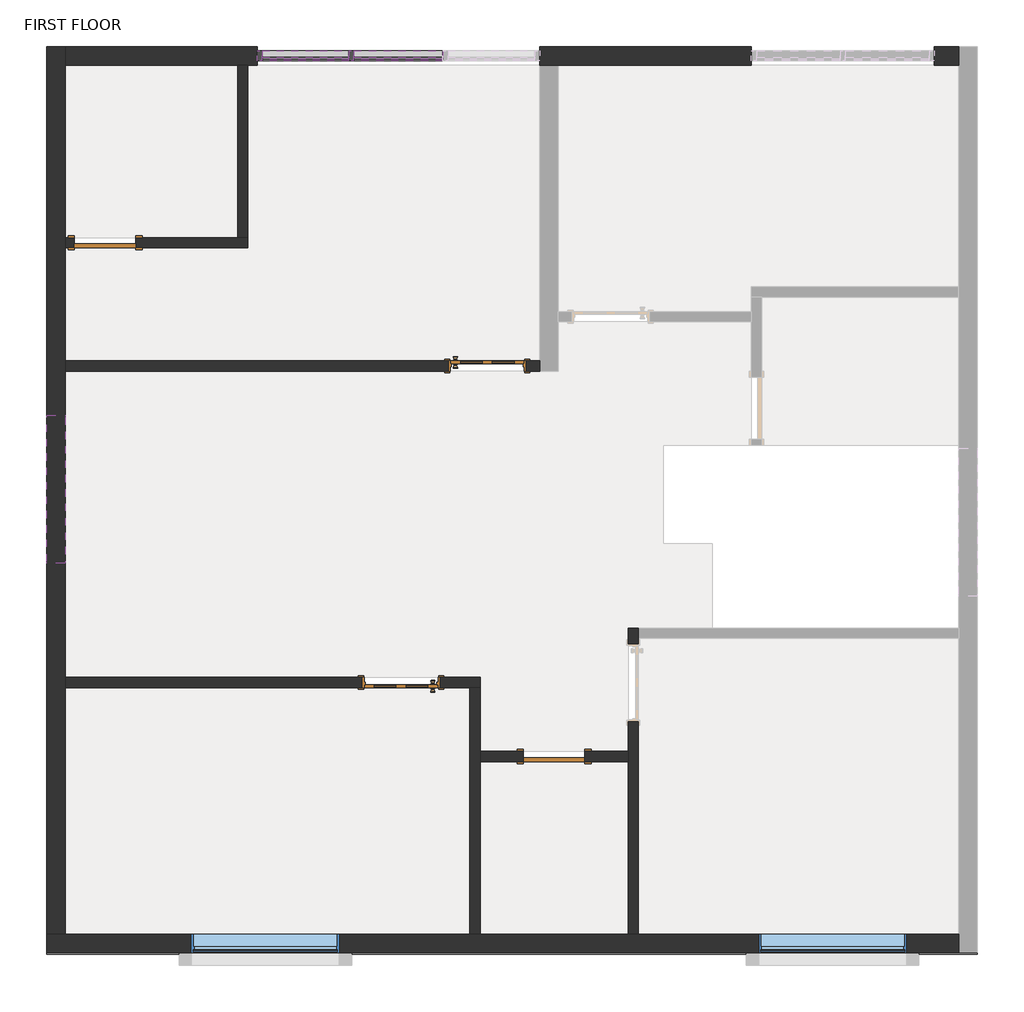
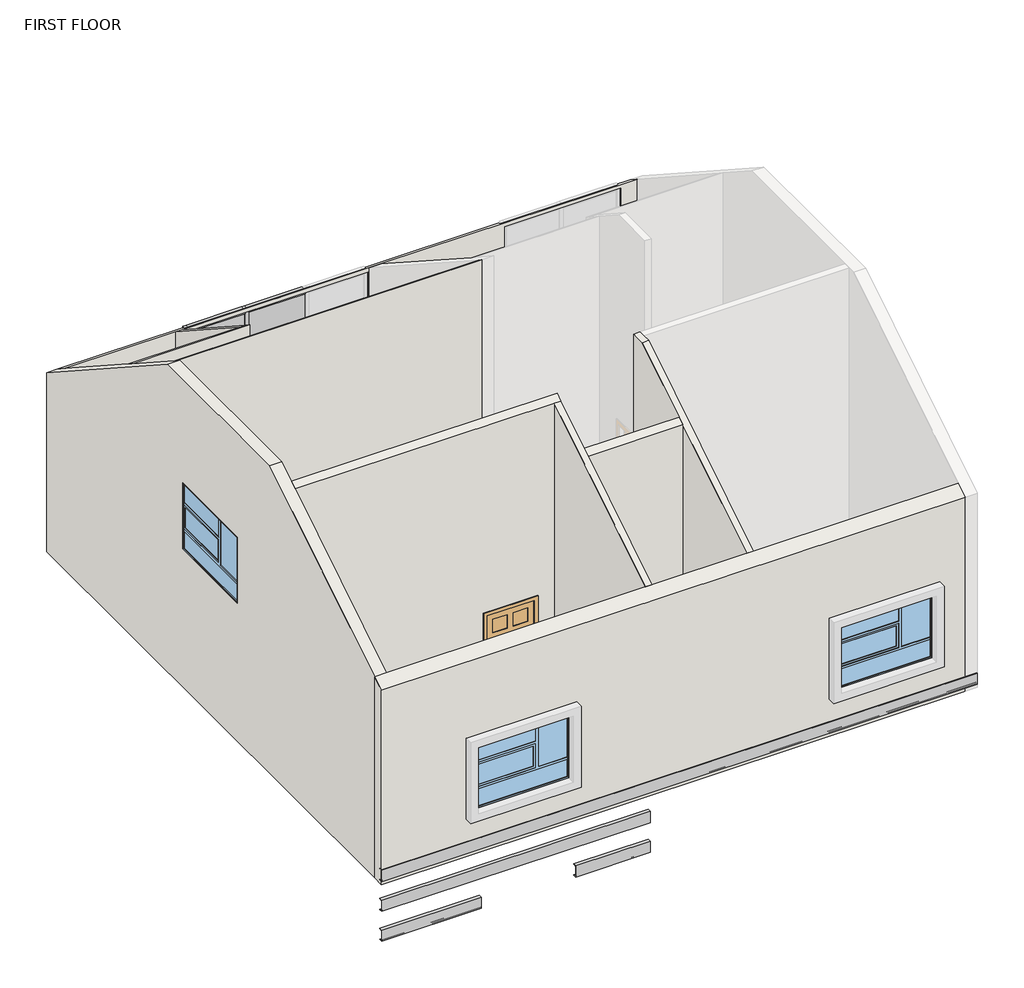
# One storey, part 1 of 2: 17 members, 10 walls, 8 plates, 4 doors, 3 proxies, 3 windows.
"""IFC4 building model written with IfcOpenShell, lengths in millimetres."""

from ifc_helpers import new_model, si_unit, point, frame, frame_2d, origin, place, context, project, spatial, polyline, circle_curve, trimmed, segment, composite_curve, outline, extrude, faceted_brep, transform, mapped, element, save
from ifc_brep_helpers import plane_surface, cylinder_surface, revolved_surface, advanced_brep
from components import door_03e3dfb5, door_1fe7f57d, member_693dcaa1, member_240932ed, member_6e77e263, member_4194b792, member_c45b528a, member_47bfaf8a, member_2b49869a, member_75074519, member_15f4dda0, member_2a4e9e33, system_panel_glazed_03e0ee66, system_panel_glazed_4b7b4477, system_panel_glazed_4d72b045, system_panel_glazed_46ac4994, system_panel_glazed_e581be51, system_panel_glazed_3a317166, system_panel_glazed_99f7726d, system_panel_glazed_de674e10, window_dd9b4f56

model = new_model("IFC4")

# Units and contexts
model_context = context("Model", 3, world=origin())
ifc_project = project(units=[si_unit("LENGTHUNIT", "METRE", prefix="MILLI")], contexts=[model_context])

# Site, building, storey
site = spatial("IfcSite", under=ifc_project)
building = spatial("IfcBuilding", under=site)
storey = spatial("IfcBuildingStorey", under=building, Name="FIRST FLOOR", Elevation=3352.8)

# Proxies
placement = place(None, origin())
element("IfcBuildingElementProxy", 1, Name="Reveal", ObjectType="Reveal", at=placement, inside=storey, context=model_context, shape_type="SweptSolid", body=[
    extrude(outline(composite_curve([segment(polyline([(-2464.7620789, 2433.713469), (-2401.5160789, 2433.713469), (-2401.5160789, 2432.3337932)]), True, "CONTINUOUS"), segment(trimmed(circle_curve(frame_2d((-2406.7611789, 2432.3337932)), 5.2451), [point((-2401.5160789, 2432.3337932))], [point((-2405.8988881, 2427.1600587))], False, "CARTESIAN"), True, "CONTINUOUS"), segment(polyline([(-2405.8988881, 2427.1600587), (-2429.5195789, 2423.223269), (-2448.7574605, 2420.016949)]), True, "CONTINUOUS"), segment(trimmed(circle_curve(frame_2d((-2447.0328789, 2409.66948)), 10.4902), [point((-2448.7574605, 2420.016949))], [point((-2457.5230789, 2409.66948))], True, "CARTESIAN"), True, "CONTINUOUS"), segment(polyline([(-2457.5230789, 2409.66948), (-2457.5230789, 2229.157458)]), True, "CONTINUOUS"), segment(trimmed(circle_curve(frame_2d((-2447.0328789, 2229.157458)), 10.4902), [point((-2457.5230789, 2229.157458))], [point((-2448.7574605, 2218.809989))], True, "CARTESIAN"), True, "CONTINUOUS"), segment(polyline([(-2448.7574605, 2218.809989), (-2429.5195789, 2215.603669), (-2405.8988881, 2211.6668793)]), True, "CONTINUOUS"), segment(trimmed(circle_curve(frame_2d((-2406.7611789, 2206.4931449)), 5.2451), [point((-2405.8988881, 2211.6668793))], [point((-2401.5160789, 2206.4931449))], False, "CARTESIAN"), True, "CONTINUOUS"), segment(polyline([(-2401.5160789, 2206.4931449), (-2401.5160789, 2205.113469), (-2464.7620789, 2205.113469), (-2464.7620789, 2433.713469)]), True, "CONTINUOUS")], self_intersect=False)), frame((-2097.5328791, 0.0, 0.0), z_axis=(1.0, 0.0, 0.0), x_axis=(0.0, 1.0, 0.0)), (0.0, 0.0, 1.0), 1435.1),
    extrude(outline(composite_curve([segment(polyline([(-2464.7620789, 2433.713469), (-2401.5160789, 2433.713469), (-2401.5160789, 2432.3337932)]), True, "CONTINUOUS"), segment(trimmed(circle_curve(frame_2d((-2406.7611789, 2432.3337932)), 5.2451), [point((-2401.5160789, 2432.3337932))], [point((-2405.8988881, 2427.1600587))], False, "CARTESIAN"), True, "CONTINUOUS"), segment(polyline([(-2405.8988881, 2427.1600587), (-2429.5195789, 2423.223269), (-2448.7574605, 2420.016949)]), True, "CONTINUOUS"), segment(trimmed(circle_curve(frame_2d((-2447.0328789, 2409.66948)), 10.4902), [point((-2448.7574605, 2420.016949))], [point((-2457.5230789, 2409.66948))], True, "CARTESIAN"), True, "CONTINUOUS"), segment(polyline([(-2457.5230789, 2409.66948), (-2457.5230789, 2229.157458)]), True, "CONTINUOUS"), segment(trimmed(circle_curve(frame_2d((-2447.0328789, 2229.157458)), 10.4902), [point((-2457.5230789, 2229.157458))], [point((-2448.7574605, 2218.809989))], True, "CARTESIAN"), True, "CONTINUOUS"), segment(polyline([(-2448.7574605, 2218.809989), (-2429.5195789, 2215.603669), (-2405.8988881, 2211.6668793)]), True, "CONTINUOUS"), segment(trimmed(circle_curve(frame_2d((-2406.7611789, 2206.4931449)), 5.2451), [point((-2405.8988881, 2211.6668793))], [point((-2401.5160789, 2206.4931449))], False, "CARTESIAN"), True, "CONTINUOUS"), segment(polyline([(-2401.5160789, 2206.4931449), (-2401.5160789, 2205.113469), (-2464.7620789, 2205.113469), (-2464.7620789, 2433.713469)]), True, "CONTINUOUS")], self_intersect=False)), frame((-5844.0328791, 0.0, 0.0), z_axis=(1.0, 0.0, 0.0), x_axis=(0.0, 1.0, 0.0)), (0.0, 0.0, 1.0), 1917.7),
])
element("IfcBuildingElementProxy", 2, Name="Reveal", ObjectType="Reveal", at=placement, inside=storey, context=model_context, shape_type="SweptSolid", body=[
    extrude(outline(composite_curve([segment(polyline([(-2464.7620789, 3043.313469), (-2401.5160789, 3043.313469), (-2401.5160789, 3041.9337932)]), True, "CONTINUOUS"), segment(trimmed(circle_curve(frame_2d((-2406.7611789, 3041.9337932)), 5.2451), [point((-2401.5160789, 3041.9337932))], [point((-2405.8988881, 3036.7600587))], False, "CARTESIAN"), True, "CONTINUOUS"), segment(polyline([(-2405.8988881, 3036.7600587), (-2429.5195789, 3032.823269), (-2448.7574605, 3029.616949)]), True, "CONTINUOUS"), segment(trimmed(circle_curve(frame_2d((-2447.0328789, 3019.26948)), 10.4902), [point((-2448.7574605, 3029.616949))], [point((-2457.5230789, 3019.26948))], True, "CARTESIAN"), True, "CONTINUOUS"), segment(polyline([(-2457.5230789, 3019.26948), (-2457.5230789, 2838.757458)]), True, "CONTINUOUS"), segment(trimmed(circle_curve(frame_2d((-2447.0328789, 2838.757458)), 10.4902), [point((-2457.5230789, 2838.757458))], [point((-2448.7574605, 2828.409989))], True, "CARTESIAN"), True, "CONTINUOUS"), segment(polyline([(-2448.7574605, 2828.409989), (-2429.5195789, 2825.203669), (-2405.8988881, 2821.2668793)]), True, "CONTINUOUS"), segment(trimmed(circle_curve(frame_2d((-2406.7611789, 2816.0931449)), 5.2451), [point((-2405.8988881, 2821.2668793))], [point((-2401.5160789, 2816.0931449))], False, "CARTESIAN"), True, "CONTINUOUS"), segment(polyline([(-2401.5160789, 2816.0931449), (-2401.5160789, 2814.713469), (-2464.7620789, 2814.713469), (-2464.7620789, 3043.313469)]), True, "CONTINUOUS")], self_intersect=False)), frame((-5844.0328791, 0.0, 0.0), z_axis=(1.0, 0.0, 0.0), x_axis=(0.0, 1.0, 0.0)), (0.0, 0.0, 1.0), 5181.6),
])
element("IfcBuildingElementProxy", 3, Name="Reveal", ObjectType="Reveal", at=placement, inside=storey, context=model_context, shape_type="SweptSolid", body=[
    extrude(outline(composite_curve([segment(polyline([(-2464.7620789, 3652.913469), (-2401.5160789, 3652.913469), (-2401.5160789, 3651.5337932)]), True, "CONTINUOUS"), segment(trimmed(circle_curve(frame_2d((-2406.7611789, 3651.5337932)), 5.2451), [point((-2401.5160789, 3651.5337932))], [point((-2405.8988881, 3646.3600587))], False, "CARTESIAN"), True, "CONTINUOUS"), segment(polyline([(-2405.8988881, 3646.3600587), (-2429.5195789, 3642.423269), (-2448.7574605, 3639.216949)]), True, "CONTINUOUS"), segment(trimmed(circle_curve(frame_2d((-2447.0328789, 3628.86948)), 10.4902), [point((-2448.7574605, 3639.216949))], [point((-2457.5230789, 3628.86948))], True, "CARTESIAN"), True, "CONTINUOUS"), segment(polyline([(-2457.5230789, 3628.86948), (-2457.5230789, 3448.357458)]), True, "CONTINUOUS"), segment(trimmed(circle_curve(frame_2d((-2447.0328789, 3448.357458)), 10.4902), [point((-2457.5230789, 3448.357458))], [point((-2448.7574605, 3438.009989))], True, "CARTESIAN"), True, "CONTINUOUS"), segment(polyline([(-2448.7574605, 3438.009989), (-2429.5195789, 3434.803669), (-2405.8988881, 3430.8668793)]), True, "CONTINUOUS"), segment(trimmed(circle_curve(frame_2d((-2406.7611789, 3425.6931449)), 5.2451), [point((-2405.8988881, 3430.8668793))], [point((-2401.5160789, 3425.6931449))], False, "CARTESIAN"), True, "CONTINUOUS"), segment(polyline([(-2401.5160789, 3425.6931449), (-2401.5160789, 3424.313469), (-2464.7620789, 3424.313469), (-2464.7620789, 3652.913469)]), True, "CONTINUOUS")], self_intersect=False)), frame((-5844.0328791, 0.0, 0.0), z_axis=(1.0, 0.0, 0.0), x_axis=(0.0, 1.0, 0.0)), (0.0, 0.0, 1.0), 11506.2),
])

# Doors
door_shape = door_03e3dfb5(model_context)
element("IfcDoor", 4, ObjectType="Door-Interior-Single-6_Panel-Wood : 36\" x 84\"", at=placement, inside=storey, context=model_context, shape_type="MappedRepresentation", body=[
    mapped(door_shape, transform((-395.7328791, 4804.9973211, 3352.8), x_axis=(1.0, 0.0, 0.0), y_axis=(0.0, 1.0, 0.0), z_axis=(0.0, 0.0, 1.0))),
])
element("IfcDoor", 5, ObjectType="Door-Interior-Single-6_Panel-Wood : 36\" x 84\"", at=placement, inside=storey, context=model_context, shape_type="MappedRepresentation", body=[
    mapped(door_shape, transform((-1462.5328791, 887.0473211, 3352.8), x_axis=(-1.0, 0.0, 0.0), y_axis=(0.0, -1.0, 0.0), z_axis=(0.0, 0.0, 1.0))),
])
door_2_shape = door_1fe7f57d(model_context)
element("IfcDoor", 6, ObjectType="Single-Flush : bathroom flush door 2' 6\" x 7'", at=placement, inside=storey, context=model_context, shape_type="MappedRepresentation", body=[
    mapped(door_2_shape, transform((-5120.1328791, 6325.8223211, 3352.8), x_axis=(-1.0, 0.0, 0.0), y_axis=(0.0, -1.0, 0.0), z_axis=(0.0, 0.0, 1.0))),
])
element("IfcDoor", 7, ObjectType="Single-Flush : bathroom flush door 2' 6\" x 7'", at=placement, inside=storey, context=model_context, shape_type="MappedRepresentation", body=[
    mapped(door_2_shape, transform((429.7671209, -24.1776789, 3352.8), x_axis=(-1.0, 0.0, 0.0), y_axis=(0.0, -1.0, 0.0), z_axis=(0.0, 0.0, 1.0))),
])

# Members
member_shape = member_693dcaa1(model_context)
element("IfcMember", 8, ObjectType="Rectangular Mullion : 2.5\" x 5\" rectangular", at=placement, inside=storey, context=model_context, shape_type="MappedRepresentation", body=[
    mapped(member_shape, transform((-3177.0328791, 8637.2223211, 7085.0688597), x_axis=(0.0, 0.0, 1.0), y_axis=(0.0, 1.0, 0.0), z_axis=(-1.0, 0.0, 0.0))),
])
member_2_shape = member_240932ed(model_context)
element("IfcMember", 9, ObjectType="Rectangular Mullion : 2.5\" x 5\" rectangular", at=placement, inside=storey, context=model_context, shape_type="MappedRepresentation", body=[
    mapped(member_2_shape, transform((-2044.6162124, 8637.2223211, 7085.0688597), x_axis=(0.0, 0.0, 1.0), y_axis=(0.0, 1.0, 0.0), z_axis=(-1.0, 0.0, 0.0))),
])
element("IfcMember", 10, ObjectType="Rectangular Mullion : 2.5\" x 5\" rectangular", at=placement, inside=storey, context=model_context, shape_type="MappedRepresentation", body=[
    mapped(member_shape, transform((-2108.1162124, 8637.2223211, 3352.8), x_axis=(0.0, 0.0, -1.0), y_axis=(0.0, 1.0, 0.0), z_axis=(1.0, 0.0, 0.0))),
])
member_3_shape = member_6e77e263(model_context)
element("IfcMember", 11, ObjectType="Rectangular Mullion : 2.5\" x 5\" rectangular", at=placement, inside=storey, context=model_context, shape_type="MappedRepresentation", body=[
    mapped(member_3_shape, transform((-2076.3662124, 8637.2223211, 3352.8), x_axis=(-1.0, 0.0, 0.0), y_axis=(0.0, 1.0, 0.0), z_axis=(0.0, 0.0, -1.0))),
])
member_4_shape = member_4194b792(model_context)
element("IfcMember", 12, ObjectType="Rectangular Mullion : 2.5\" x 5\" rectangular", at=placement, inside=storey, context=model_context, shape_type="MappedRepresentation", body=[
    mapped(member_4_shape, transform((-3177.0328791, 8637.2223211, 3962.4), x_axis=(0.0, 0.0, 1.0), y_axis=(0.0, 1.0, 0.0), z_axis=(-1.0, 0.0, 0.0))),
])
element("IfcMember", 13, ObjectType="Rectangular Mullion : 2.5\" x 5\" rectangular", at=placement, inside=storey, context=model_context, shape_type="MappedRepresentation", body=[
    mapped(member_4_shape, transform((-3177.0328791, 8637.2223211, 5181.6), x_axis=(0.0, 0.0, 1.0), y_axis=(0.0, 1.0, 0.0), z_axis=(-1.0, 0.0, 0.0))),
])
element("IfcMember", 14, ObjectType="Rectangular Mullion : 2.5\" x 5\" rectangular", at=placement, inside=storey, context=model_context, shape_type="MappedRepresentation", body=[
    mapped(member_4_shape, transform((-3177.0328791, 8637.2223211, 5791.2), x_axis=(0.0, 0.0, 1.0), y_axis=(0.0, 1.0, 0.0), z_axis=(-1.0, 0.0, 0.0))),
])
member_5_shape = member_c45b528a(model_context)
element("IfcMember", 15, ObjectType="Rectangular Mullion : 2.5\" x 5\" rectangular", at=placement, inside=storey, context=model_context, shape_type="MappedRepresentation", body=[
    mapped(member_5_shape, transform((-2044.6162124, 8637.2223211, 3962.4), x_axis=(0.0, 0.0, 1.0), y_axis=(0.0, 1.0, 0.0), z_axis=(-1.0, 0.0, 0.0))),
])
element("IfcMember", 16, ObjectType="Rectangular Mullion : 2.5\" x 5\" rectangular", at=placement, inside=storey, context=model_context, shape_type="MappedRepresentation", body=[
    mapped(member_5_shape, transform((-2044.6162124, 8637.2223211, 5181.6), x_axis=(0.0, 0.0, 1.0), y_axis=(0.0, 1.0, 0.0), z_axis=(-1.0, 0.0, 0.0))),
])
element("IfcMember", 17, ObjectType="Rectangular Mullion : 2.5\" x 5\" rectangular", at=placement, inside=storey, context=model_context, shape_type="MappedRepresentation", body=[
    mapped(member_5_shape, transform((-2044.6162124, 8637.2223211, 5791.2), x_axis=(0.0, 0.0, 1.0), y_axis=(0.0, 1.0, 0.0), z_axis=(-1.0, 0.0, 0.0))),
])
member_6_shape = member_47bfaf8a(model_context)
element("IfcMember", 18, ObjectType="Rectangular Mullion : 2.5\" x 5\" rectangular", at=placement, inside=storey, context=model_context, shape_type="MappedRepresentation", body=[
    mapped(member_6_shape, transform((-3240.5328791, 8637.2223211, 3352.8), x_axis=(-1.0, 0.0, 0.0), y_axis=(0.0, 1.0, 0.0), z_axis=(0.0, 0.0, -1.0))),
])
member_7_shape = member_2b49869a(model_context)
element("IfcMember", 19, ObjectType="Rectangular Mullion : 2.5\" x 5\" rectangular", at=placement, inside=storey, context=model_context, shape_type="MappedRepresentation", body=[
    mapped(member_7_shape, transform((-2076.3662124, 8637.2223211, 3962.4), x_axis=(-1.0, 0.0, 0.0), y_axis=(0.0, 1.0, 0.0), z_axis=(0.0, 0.0, -1.0))),
])
member_8_shape = member_75074519(model_context)
element("IfcMember", 20, ObjectType="Rectangular Mullion : 2.5\" x 5\" rectangular", at=placement, inside=storey, context=model_context, shape_type="MappedRepresentation", body=[
    mapped(member_8_shape, transform((-3240.5328791, 8637.2223211, 3962.4), x_axis=(-1.0, 0.0, 0.0), y_axis=(0.0, 1.0, 0.0), z_axis=(0.0, 0.0, -1.0))),
])
element("IfcMember", 21, ObjectType="Rectangular Mullion : 2.5\" x 5\" rectangular", at=placement, inside=storey, context=model_context, shape_type="MappedRepresentation", body=[
    mapped(member_3_shape, transform((-2076.3662124, 8637.2223211, 5181.6), x_axis=(-1.0, 0.0, 0.0), y_axis=(0.0, 1.0, 0.0), z_axis=(0.0, 0.0, -1.0))),
])
element("IfcMember", 22, ObjectType="Rectangular Mullion : 2.5\" x 5\" rectangular", at=placement, inside=storey, context=model_context, shape_type="MappedRepresentation", body=[
    mapped(member_6_shape, transform((-3240.5328791, 8637.2223211, 5181.6), x_axis=(-1.0, 0.0, 0.0), y_axis=(0.0, 1.0, 0.0), z_axis=(0.0, 0.0, -1.0))),
])
member_9_shape = member_15f4dda0(model_context)
element("IfcMember", 23, ObjectType="Rectangular Mullion : 2.5\" x 5\" rectangular", at=placement, inside=storey, context=model_context, shape_type="MappedRepresentation", body=[
    mapped(member_9_shape, transform((-2076.3662124, 8637.2223211, 5791.2), x_axis=(-1.0, 0.0, 0.0), y_axis=(0.0, 1.0, 0.0), z_axis=(0.0, 0.0, -1.0))),
])
member_10_shape = member_2a4e9e33(model_context)
element("IfcMember", 24, ObjectType="Rectangular Mullion : 2.5\" x 5\" rectangular", at=placement, inside=storey, context=model_context, shape_type="MappedRepresentation", body=[
    mapped(member_10_shape, transform((-3240.5328791, 8637.2223211, 5791.2), x_axis=(-1.0, 0.0, 0.0), y_axis=(0.0, 1.0, 0.0), z_axis=(0.0, 0.0, -1.0))),
])

# Plates
system_panel_glazed_shape = system_panel_glazed_03e0ee66(model_context)
element("IfcPlate", 25, ObjectType="System Panel : Glazed", at=placement, inside=storey, context=model_context, shape_type="MappedRepresentation", body=[
    mapped(system_panel_glazed_shape, transform((-2642.5745458, 8637.2223211, 3416.3), x_axis=(-1.0, 0.0, 0.0), y_axis=(0.0, -1.0, 0.0), z_axis=(0.0, 0.0, 1.0))),
])
system_panel_glazed_2_shape = system_panel_glazed_4b7b4477(model_context)
element("IfcPlate", 26, ObjectType="System Panel : Glazed", at=placement, inside=storey, context=model_context, shape_type="MappedRepresentation", body=[
    mapped(system_panel_glazed_2_shape, transform((-1494.2828791, 8637.2223211, 3416.3), x_axis=(-1.0, 0.0, 0.0), y_axis=(0.0, -1.0, 0.0), z_axis=(0.0, 0.0, 1.0))),
])
system_panel_glazed_3_shape = system_panel_glazed_4d72b045(model_context)
element("IfcPlate", 27, ObjectType="System Panel : Glazed", at=placement, inside=storey, context=model_context, shape_type="MappedRepresentation", body=[
    mapped(system_panel_glazed_3_shape, transform((-1494.2828791, 8637.2223211, 3994.15), x_axis=(-1.0, 0.0, 0.0), y_axis=(0.0, -1.0, 0.0), z_axis=(0.0, 0.0, 1.0))),
])
system_panel_glazed_4_shape = system_panel_glazed_46ac4994(model_context)
element("IfcPlate", 28, ObjectType="System Panel : Glazed", at=placement, inside=storey, context=model_context, shape_type="MappedRepresentation", body=[
    mapped(system_panel_glazed_4_shape, transform((-2642.5745458, 8637.2223211, 3994.15), x_axis=(-1.0, 0.0, 0.0), y_axis=(0.0, -1.0, 0.0), z_axis=(0.0, 0.0, 1.0))),
])
system_panel_glazed_5_shape = system_panel_glazed_e581be51(model_context)
element("IfcPlate", 29, ObjectType="System Panel : Glazed", at=placement, inside=storey, context=model_context, shape_type="MappedRepresentation", body=[
    mapped(system_panel_glazed_5_shape, transform((-2642.5745458, 8637.2223211, 5213.35), x_axis=(-1.0, 0.0, 0.0), y_axis=(0.0, -1.0, 0.0), z_axis=(0.0, 0.0, 1.0))),
])
system_panel_glazed_6_shape = system_panel_glazed_3a317166(model_context)
element("IfcPlate", 30, ObjectType="System Panel : Glazed", at=placement, inside=storey, context=model_context, shape_type="MappedRepresentation", body=[
    mapped(system_panel_glazed_6_shape, transform((-1494.2828791, 8637.2223211, 5213.35), x_axis=(-1.0, 0.0, 0.0), y_axis=(0.0, -1.0, 0.0), z_axis=(0.0, 0.0, 1.0))),
])
system_panel_glazed_7_shape = system_panel_glazed_99f7726d(model_context)
element("IfcPlate", 31, ObjectType="System Panel : Glazed", at=placement, inside=storey, context=model_context, shape_type="MappedRepresentation", body=[
    mapped(system_panel_glazed_7_shape, transform((-2642.5745458, 8637.2223211, 5822.95), x_axis=(-1.0, 0.0, 0.0), y_axis=(0.0, -1.0, 0.0), z_axis=(0.0, 0.0, 1.0))),
])
system_panel_glazed_8_shape = system_panel_glazed_de674e10(model_context)
element("IfcPlate", 32, ObjectType="System Panel : Glazed", at=placement, inside=storey, context=model_context, shape_type="MappedRepresentation", body=[
    mapped(system_panel_glazed_8_shape, transform((-1494.2828791, 8637.2223211, 5822.95), x_axis=(-1.0, 0.0, 0.0), y_axis=(0.0, -1.0, 0.0), z_axis=(0.0, 0.0, 1.0))),
])

# Walls
element("IfcWall", 33, ObjectType="INNER WALL 5\"", at=placement, inside=storey, context=model_context, shape_type="Brep", body=[
    faceted_brep([(-5615.4328791, 6262.3223211, 3352.8), (-5501.1328791, 6262.3223211, 3352.8), (-5501.1328791, 6262.3223211, 5384.8), (-4739.1328791, 6262.3223211, 5384.8), (-4739.1328791, 6262.3223211, 3352.8), (-3354.8328791, 6262.3223211, 3352.8), (-3354.8328791, 6262.3223211, 8627.3469528), (-5615.4328791, 6262.3223211, 8627.3469528), (-5501.1328791, 6389.3223211, 5384.8), (-5501.1328791, 6389.3223211, 3352.8), (-5615.4328791, 6389.3223211, 3352.8), (-5615.4328791, 6389.3223211, 8544.8721884), (-3481.8328791, 6389.3223211, 8544.8721884), (-3354.8328791, 6389.3223211, 8544.8721884), (-3354.8328791, 6389.3223211, 3352.8), (-3481.8328791, 6389.3223211, 3352.8), (-4739.1328791, 6389.3223211, 3352.8), (-4739.1328791, 6389.3223211, 5384.8)], [[[0, 1, 2, 3, 4, 5, 6, 7]], [[8, 9, 10, 11, 12, 13, 14, 15, 16, 17]], [[10, 9, 1, 0]], [[16, 15, 14, 5, 4]], [[0, 7, 11, 10]], [[6, 5, 14, 13]], [[2, 1, 9, 8]], [[3, 2, 8, 17]], [[4, 3, 17, 16]], [[7, 6, 13, 12, 11]]]),
])
element("IfcWall", 34, ObjectType="INNER WALL 5\"", at=placement, inside=storey, context=model_context, shape_type="SweptSolid", body=[
    extrude(outline(polyline([(6389.3223211, 3352.8), (6389.3223211, 8544.8721884), (8522.9223211, 7159.2961476), (8522.9223211, 3352.8), (6389.3223211, 3352.8)])), frame((-3481.8328791, 0.0, 0.0), z_axis=(1.0, 0.0, 0.0), x_axis=(0.0, 1.0, 0.0)), (0.0, 0.0, 1.0), 127.0),
])
element("IfcWall", 35, ObjectType="INNER WALL 5\"", at=placement, inside=storey, context=model_context, shape_type="Brep", body=[
    faceted_brep([(251.9671209, 4738.3223211, 3352.8), (251.9671209, 4738.3223211, 9617.0441248), (-5615.4328791, 4738.3223211, 9617.0441248), (-5615.4328791, 4738.3223211, 3352.8), (-878.3328791, 4738.3223211, 3352.8), (-878.3328791, 4738.3223211, 5511.8), (86.8671209, 4738.3223211, 5511.8), (86.8671209, 4738.3223211, 3352.8), (251.9671209, 4865.3223211, 9534.5693605), (251.9671209, 4865.3223211, 3352.8), (86.8671209, 4865.3223211, 3352.8), (86.8671209, 4865.3223211, 5511.8), (-878.3328791, 4865.3223211, 5511.8), (-878.3328791, 4865.3223211, 3352.8), (-5615.4328791, 4865.3223211, 3352.8), (-5615.4328791, 4865.3223211, 9534.5693605)], [[[0, 1, 2, 3, 4, 5, 6, 7]], [[8, 9, 10, 11, 12, 13, 14, 15]], [[3, 14, 13, 4]], [[9, 0, 7, 10]], [[1, 0, 9, 8]], [[3, 2, 15, 14]], [[6, 11, 10, 7]], [[11, 6, 5, 12]], [[12, 5, 4, 13]], [[2, 1, 8, 15]]]),
])
element("IfcWall", 36, ObjectType="INNER WALL 5\"", at=placement, inside=storey, context=model_context, shape_type="Brep", body=[
    faceted_brep([(1471.1671209, -2221.2776789, 7460.5048127), (1471.1671209, -2221.2776789, 3352.8), (1471.1671209, 407.6223211, 3352.8), (1471.1671209, 407.6223211, 5511.8), (1471.1671209, 1372.8223211, 5511.8), (1471.1671209, 1372.8223211, 3352.8), (1471.1671209, 1436.3223211, 3352.8), (1471.1671209, 1563.3223211, 3352.8), (1471.1671209, 1563.3223211, 9646.3602906), (1471.1671209, 1436.3223211, 9646.3602906), (1471.1671209, 1276.8223179, 9646.3602906), (1344.1671209, -2221.2776789, 3352.8), (1344.1671209, -2221.2776789, 7460.5048127), (1344.1671209, -87.6776789, 8793.726062), (1344.1671209, 39.3223211, 8873.0844697), (1344.1671209, 1276.8223179, 9646.3602906), (1344.1671209, 1563.3223211, 9646.3602906), (1344.1671209, 1563.3223211, 3352.8), (1344.1671209, 1372.8223211, 3352.8), (1344.1671209, 1372.8223211, 5511.8), (1344.1671209, 407.6223211, 5511.8), (1344.1671209, 407.6223211, 3352.8), (1344.1671209, 39.3223211, 3352.8), (1344.1671209, -87.6776789, 3352.8)], [[[0, 1, 2, 3, 4, 5, 6, 7, 8, 9, 10]], [[11, 12, 13, 14, 15, 16, 17, 18, 19, 20, 21, 22, 23]], [[1, 11, 23, 22, 21, 2]], [[17, 7, 6, 5, 18]], [[1, 0, 12, 11]], [[8, 7, 17, 16]], [[20, 3, 2, 21]], [[3, 20, 19, 4]], [[4, 19, 18, 5]], [[12, 0, 10, 15, 14, 13]], [[8, 16, 15, 10, 9]]]),
])
element("IfcWall", 37, ObjectType="INNER WALL 5\"", at=placement, inside=storey, context=model_context, shape_type="Brep", body=[
    faceted_brep([(-5615.4328791, 826.7223211, 9365.1065974), (-5615.4328791, 826.7223211, 3352.8), (-1945.1328791, 826.7223211, 3352.8), (-1945.1328791, 826.7223211, 5511.8), (-979.9328791, 826.7223211, 5511.8), (-979.9328791, 826.7223211, 3352.8), (-611.6328791, 826.7223211, 3352.8), (-484.6328791, 826.7223211, 3352.8), (-484.6328791, 826.7223211, 9365.1065974), (-611.6328791, 826.7223211, 9365.1065974), (-5615.4328791, 953.7223211, 3352.8), (-5615.4328791, 953.7223211, 9444.4650051), (-484.6328791, 953.7223211, 9444.4650051), (-484.6328791, 953.7223211, 3352.8), (-979.9328791, 953.7223211, 3352.8), (-979.9328791, 953.7223211, 5511.8), (-1945.1328791, 953.7223211, 5511.8), (-1945.1328791, 953.7223211, 3352.8)], [[[0, 1, 2, 3, 4, 5, 6, 7, 8, 9]], [[10, 11, 12, 13, 14, 15, 16, 17]], [[1, 10, 17, 2]], [[13, 7, 6, 5, 14]], [[1, 0, 11, 10]], [[8, 7, 13, 12]], [[16, 3, 2, 17]], [[3, 16, 15, 4]], [[4, 15, 14, 5]], [[0, 9, 8, 12, 11]]]),
])
element("IfcWall", 38, ObjectType="INNER WALL 5\"", at=placement, inside=storey, context=model_context, shape_type="Brep", body=[
    faceted_brep([(-611.6328791, 826.7223211, 3352.8), (-611.6328791, -2221.2776789, 3352.8), (-611.6328791, -2221.2776789, 7460.5048127), (-611.6328791, 826.7223211, 9365.1065974), (-484.6328791, 826.7223211, 3352.8), (-484.6328791, 826.7223211, 9365.1065974), (-484.6328791, 39.3223211, 8873.0844697), (-484.6328791, -87.6776789, 8793.726062), (-484.6328791, -2221.2776789, 7460.5048127), (-484.6328791, -2221.2776789, 3352.8), (-484.6328791, -87.6776789, 3352.8), (-484.6328791, 39.3223211, 3352.8)], [[[0, 1, 2, 3]], [[4, 5, 6, 7, 8, 9, 10, 11]], [[1, 0, 4, 11, 10, 9]], [[0, 3, 5, 4]], [[2, 1, 9, 8]], [[3, 2, 8, 7, 6, 5]]]),
])
element("IfcWall", 39, ObjectType="INNER WALL 5\"", at=placement, inside=storey, context=model_context, shape_type="Brep", body=[
    faceted_brep([(-484.6328791, -87.6776789, 3352.8), (48.7671209, -87.6776789, 3352.8), (48.7671209, -87.6776789, 5384.8), (810.7671209, -87.6776789, 5384.8), (810.7671209, -87.6776789, 3352.8), (1344.1671209, -87.6776789, 3352.8), (1344.1671209, -87.6776789, 8793.726062), (-484.6328791, -87.6776789, 8793.726062), (48.7671209, 39.3223211, 5384.8), (48.7671209, 39.3223211, 3352.8), (-484.6328791, 39.3223211, 3352.8), (-484.6328791, 39.3223211, 8873.0844697), (1344.1671209, 39.3223211, 8873.0844697), (1344.1671209, 39.3223211, 3352.8), (810.7671209, 39.3223211, 3352.8), (810.7671209, 39.3223211, 5384.8)], [[[0, 1, 2, 3, 4, 5, 6, 7]], [[8, 9, 10, 11, 12, 13, 14, 15]], [[14, 13, 5, 4]], [[10, 9, 1, 0]], [[6, 5, 13, 12]], [[0, 7, 11, 10]], [[2, 1, 9, 8]], [[3, 2, 8, 15]], [[4, 3, 15, 14]], [[7, 6, 12, 11]]]),
])
element("IfcWall", 40, ObjectType="OUTER WALL 9\"", at=placement, inside=storey, context=model_context, shape_type="AdvancedBrep", body=[
    advanced_brep(
    [(5433.5671209, -2221.2776789, 3352.8), (1471.1671209, -2221.2776789, 3352.8), (1344.1671209, -2221.2776789, 3352.8), (-484.6328791, -2221.2776789, 3352.8), (-611.6328791, -2221.2776789, 3352.8), (-5615.4328791, -2221.2776789, 3352.8), (-5844.0328791, -2221.2776789, 3352.8), (-5844.0328791, -2221.2776789, 7460.5048127), (-5615.4328791, -2221.2776789, 7460.5048127), (-611.6328791, -2221.2776789, 7460.5048127), (-484.6328791, -2221.2776789, 7460.5048127), (1344.1671209, -2221.2776789, 7460.5048127), (1471.1671209, -2221.2776789, 7460.5048127), (5433.5671209, -2221.2776789, 7460.5048127), (-4053.3328791, -2221.2776789, 5613.4), (-4053.3328791, -2221.2776789, 4267.2), (-2224.5328791, -2221.2776789, 4267.2), (-2224.5328791, -2221.2776789, 5613.4), (2957.0671209, -2221.2776789, 5613.4), (2957.0671209, -2221.2776789, 4267.2), (4785.8671209, -2221.2776789, 4267.2), (4785.8671209, -2221.2776789, 5613.4), (-5844.0328791, -2449.8776789, 3352.8), (5433.5671209, -2449.8776789, 3352.8), (5433.5671209, -2449.8776789, 3424.313469), (-5844.0328791, -2449.8776789, 3424.313469), (5433.5671209, -2449.8776789, 7317.6596789), (-5844.0328791, -2449.8776789, 7317.6596789), (-5844.0328791, -2449.8776789, 3652.913469), (5433.5671209, -2449.8776789, 3652.913469), (-4053.3328791, -2449.8776789, 4267.2), (-4053.3328791, -2449.8776789, 5613.4), (-2224.5328791, -2449.8776789, 5613.4), (-2224.5328791, -2449.8776789, 4267.2), (2957.0671209, -2449.8776789, 4267.2), (2957.0671209, -2449.8776789, 5613.4), (4785.8671209, -2449.8776789, 5613.4), (4785.8671209, -2449.8776789, 4267.2), (5433.5671209, -2449.8776789, 3438.260359), (5433.5671209, -2449.8776789, 3638.9665791), (-5844.0328791, -2449.8776789, 3638.9665791), (-5844.0328791, -2449.8776789, 3438.260359), (5433.5671209, -2401.5160789, 3652.913469), (5433.5671209, -2401.5160789, 3651.5337932), (5433.5671209, -2405.8988881, 3646.3600587), (5433.5671209, -2448.7574605, 3639.216949), (5433.5671209, -2448.7574605, 3438.009989), (5433.5671209, -2405.8988881, 3430.8668793), (5433.5671209, -2401.5160789, 3425.6931449), (5433.5671209, -2401.5160789, 3424.313469), (-5844.0328791, -2401.5160789, 3424.313469), (-5844.0328791, -2401.5160789, 3425.6931449), (-5844.0328791, -2405.8988881, 3430.8668793), (-5844.0328791, -2448.7574605, 3438.009989), (-5844.0328791, -2448.7574605, 3639.216949), (-5844.0328791, -2405.8988881, 3646.3600587), (-5844.0328791, -2401.5160789, 3651.5337932), (-5844.0328791, -2401.5160789, 3652.913469)],
    [
        (0, 1),
        (1, 2),
        (2, 3),
        (3, 4),
        (4, 5),
        (5, 6),
        (6, 7),
        (7, 8),
        (8, 9),
        (9, 10),
        (10, 11),
        (11, 12),
        (12, 13),
        (13, 0),
        (14, 15),
        (15, 16),
        (16, 17),
        (17, 14),
        (18, 19),
        (19, 20),
        (20, 21),
        (21, 18),
        (22, 23),
        (23, 24),
        (24, 25),
        (25, 22),
        (26, 27),
        (27, 28),
        (28, 29),
        (29, 26),
        (30, 31),
        (31, 32),
        (32, 33),
        (33, 30),
        (34, 35),
        (35, 36),
        (36, 37),
        (37, 34),
        (38, 39),
        (39, 40),
        (40, 41),
        (41, 38),
        (0, 23),
        (22, 6),
        (13, 26),
        (29, 42),
        (42, 43),
        (43, 44, circle_curve(frame((5433.5671209, -2406.7611789, 3651.5337932), z_axis=(-1.0, 0.0, 0.0), x_axis=(0.0, 1.0, 0.0)), 5.2451)),
        (44, 45),
        (45, 39, circle_curve(frame((5433.5671209, -2447.0328789, 3628.86948), z_axis=(1.0, 0.0, 0.0), x_axis=(0.0, 1.0, 0.0)), 10.4902)),
        (38, 46, circle_curve(frame((5433.5671209, -2447.0328789, 3448.357458), z_axis=(1.0, 0.0, 0.0), x_axis=(0.0, 1.0, 0.0)), 10.4902)),
        (46, 47),
        (47, 48, circle_curve(frame((5433.5671209, -2406.7611789, 3425.6931449), z_axis=(-1.0, 0.0, 0.0), x_axis=(0.0, 1.0, 0.0)), 5.2451)),
        (48, 49),
        (49, 24),
        (25, 50),
        (50, 51),
        (51, 52, circle_curve(frame((-5844.0328791, -2406.7611789, 3425.6931449), z_axis=(1.0, 0.0, 0.0), x_axis=(0.0, 1.0, 0.0)), 5.2451)),
        (52, 53),
        (53, 41, circle_curve(frame((-5844.0328791, -2447.0328789, 3448.357458), z_axis=(-1.0, 0.0, 0.0), x_axis=(0.0, 1.0, 0.0)), 10.4902)),
        (40, 54, circle_curve(frame((-5844.0328791, -2447.0328789, 3628.86948), z_axis=(-1.0, 0.0, 0.0), x_axis=(0.0, 1.0, 0.0)), 10.4902)),
        (54, 55),
        (55, 56, circle_curve(frame((-5844.0328791, -2406.7611789, 3651.5337932), z_axis=(1.0, 0.0, 0.0), x_axis=(0.0, 1.0, 0.0)), 5.2451)),
        (56, 57),
        (57, 28),
        (27, 7),
        (14, 31),
        (30, 15),
        (33, 16),
        (32, 17),
        (18, 35),
        (34, 19),
        (37, 20),
        (36, 21),
        (49, 50),
        (48, 51),
        (47, 52),
        (46, 53),
        (45, 54),
        (44, 55),
        (43, 56),
        (42, 57),
    ],
    [
        plane_surface(frame((5662.1671209, -2221.2776789, 3352.8), z_axis=(0.0, 1.0, 0.0), x_axis=(-1.0, 0.0, 0.0))),
        plane_surface(frame((5662.1671209, -2449.8776789, 3352.8), z_axis=(0.0, -1.0, 0.0), x_axis=(1.0, 0.0, 0.0))),
        plane_surface(frame((5547.8671209, -2221.2776789, 3352.8), z_axis=(0.0, 0.0, -1.0), x_axis=(0.0, -1.0, 0.0))),
        plane_surface(frame((5433.5671209, 8740.4868082, 3352.8), z_axis=(1.0, 0.0, 0.0), x_axis=(0.0, -1.0, 0.0))),
        plane_surface(frame((-5844.0328791, -2449.8776789, 3352.8), z_axis=(-1.0, 0.0, 0.0), x_axis=(0.0, -1.0, 0.0))),
        plane_surface(frame((-4053.3328791, -2221.2776789, 5613.4), z_axis=(1.0, 0.0, 0.0), x_axis=(0.0, -1.0, 0.0))),
        plane_surface(frame((-4053.3328791, -2221.2776789, 4267.2), z_axis=(0.0, 0.0, 1.0), x_axis=(0.0, -1.0, 0.0))),
        plane_surface(frame((-2224.5328791, -2221.2776789, 4267.2), z_axis=(-1.0, 0.0, 0.0), x_axis=(0.0, -1.0, 0.0))),
        plane_surface(frame((-2224.5328791, -2221.2776789, 5613.4), z_axis=(0.0, 0.0, -1.0), x_axis=(0.0, -1.0, 0.0))),
        plane_surface(frame((2957.0671209, -2221.2776789, 5613.4), z_axis=(1.0, 0.0, 0.0), x_axis=(0.0, -1.0, 0.0))),
        plane_surface(frame((2957.0671209, -2221.2776789, 4267.2), z_axis=(0.0, 0.0, 1.0), x_axis=(0.0, -1.0, 0.0))),
        plane_surface(frame((4785.8671209, -2221.2776789, 4267.2), z_axis=(-1.0, 0.0, 0.0), x_axis=(0.0, -1.0, 0.0))),
        plane_surface(frame((4785.8671209, -2221.2776789, 5613.4), z_axis=(0.0, 0.0, -1.0), x_axis=(0.0, -1.0, 0.0))),
        plane_surface(frame((-5844.0328791, 1276.8223179, 9646.3602906), z_axis=(0.0, -0.5299192642332075, 0.8480480961564245), x_axis=(1.0, 0.0, 0.0))),
        plane_surface(frame((5662.1671209, -2464.7620789, 3424.313469), z_axis=(0.0, 0.0, 1.0), x_axis=(-1.0, 0.0, 0.0))),
        plane_surface(frame((5662.1671209, -2401.5160789, 3424.313469), z_axis=(0.0, -1.0, 0.0), x_axis=(-1.0, 0.0, 0.0))),
        revolved_surface(polyline([(5433.5671209, -2401.5160788999997, 3425.6931449), (-5844.032879100001, -2401.5160788999997, 3425.6931449)]), (5662.1671209, -2406.7611789, 3425.6931449), (1.0, 0.0, 0.0)),
        plane_surface(frame((5662.1671209, -2429.5195789, 3434.803669), z_axis=(0.0, -0.1643993072168769, -0.9863938705135039), x_axis=(-1.0, 0.0, 0.0))),
        cylinder_surface(frame((5662.1671209, -2447.0328789, 3448.357458), z_axis=(-1.0, 0.0, 0.0), x_axis=(0.0, 1.0, 0.0)), 10.4902),
        cylinder_surface(frame((5662.1671209, -2447.0328789, 3628.86948), z_axis=(-1.0, 0.0, 0.0), x_axis=(0.0, 1.0, 0.0)), 10.4902),
        plane_surface(frame((5662.1671209, -2429.5195789, 3642.423269), z_axis=(0.0, -0.16439930721687082, 0.9863938705135049), x_axis=(-1.0, 0.0, 0.0))),
        revolved_surface(polyline([(5433.5671209, -2401.5160788999997, 3651.5337932), (-5844.032879100001, -2401.5160788999997, 3651.5337932)]), (5662.1671209, -2406.7611789, 3651.5337932), (1.0, 0.0, 0.0)),
        plane_surface(frame((5662.1671209, -2401.5160789, 3651.5337932), z_axis=(0.0, -1.0, 0.0), x_axis=(-1.0, 0.0, 0.0))),
        plane_surface(frame((5662.1671209, -2401.5160789, 3652.913469), z_axis=(0.0, 0.0, -1.0), x_axis=(-1.0, 0.0, 0.0))),
    ],
    [
        (0, [[1, 2, 3, 4, 5, 6, 7, 8, 9, 10, 11, 12, 13, 14], [15, 16, 17, 18], [19, 20, 21, 22]]),
        (1, [[23, 24, 25, 26]]),
        (1, [[27, 28, 29, 30], [31, 32, 33, 34], [35, 36, 37, 38]]),
        (1, [[39, 40, 41, 42]]),
        (2, [[-6, -5, -4, -3, -2, -1, 43, -23, 44]]),
        (3, [[-14, 45, -30, 46, 47, 48, 49, 50, -39, 51, 52, 53, 54, 55, -24, -43]]),
        (4, [[-7, -44, -26, 56, 57, 58, 59, 60, -41, 61, 62, 63, 64, 65, -28, 66]]),
        (5, [[-15, 67, -31, 68]]),
        (6, [[-16, -68, -34, 69]]),
        (7, [[-17, -69, -33, 70]]),
        (8, [[-18, -70, -32, -67]]),
        (9, [[-19, 71, -35, 72]]),
        (10, [[-20, -72, -38, 73]]),
        (11, [[-21, -73, -37, 74]]),
        (12, [[-22, -74, -36, -71]]),
        (13, [[-13, -12, -11, -10, -9, -8, -66, -27, -45]]),
        (14, [[75, -56, -25, -55]]),
        (15, [[-75, -54, 76, -57]]),
        (16, [[-76, -53, 77, -58]]),
        (17, [[-77, -52, 78, -59]]),
        (18, [[-78, -51, -42, -60]]),
        (19, [[79, -61, -40, -50]]),
        (20, [[-79, -49, 80, -62]]),
        (21, [[-80, -48, 81, -63]]),
        (22, [[-81, -47, 82, -64]]),
        (23, [[-82, -46, -29, -65]]),
    ],
),
])
element("IfcWall", 41, ObjectType="OUTER WALL 9\"", at=placement, inside=storey, context=model_context, shape_type="Brep", body=[
    faceted_brep([(-5615.4328791, -2221.2776789, 3352.8), (-5615.4328791, 826.7223211, 3352.8), (-5615.4328791, 953.7223211, 3352.8), (-5615.4328791, 4738.3223211, 3352.8), (-5615.4328791, 4865.3223211, 3352.8), (-5615.4328791, 6262.3223211, 3352.8), (-5615.4328791, 6389.3223211, 3352.8), (-5615.4328791, 8522.9223211, 3352.8), (-5615.4328791, 8751.5223211, 3352.8), (-5615.4328791, 8751.5223211, 7010.8415718), (-5615.4328791, 8522.9223211, 7159.2961476), (-5615.4328791, 6389.3223211, 8544.8721884), (-5615.4328791, 6262.3223211, 8627.3469528), (-5615.4328791, 4865.3223211, 9534.5693605), (-5615.4328791, 4738.3223211, 9617.0441248), (-5615.4328791, 4693.1793845, 9646.3602906), (-5615.4328791, 1276.8223179, 9646.3602906), (-5615.4328791, 953.7223211, 9444.4650051), (-5615.4328791, 826.7223211, 9365.1065974), (-5615.4328791, -2221.2776789, 7460.5048127), (-5615.4328791, 4192.2223211, 7526.6456568), (-5615.4328791, 4192.2223211, 6180.4456568), (-5615.4328791, 2363.4223211, 6180.4456568), (-5615.4328791, 2363.4223211, 7526.6456568), (-5844.0328791, -2221.2776789, 3352.8), (-5844.0328791, -2221.2776789, 7460.5048127), (-5844.0328791, 1276.8223179, 9646.3602906), (-5844.0328791, 4693.1793845, 9646.3602906), (-5844.0328791, 8751.5223211, 7010.8415718), (-5844.0328791, 8751.5223211, 3352.8), (-5844.0328791, 4192.2223211, 7526.6456568), (-5844.0328791, 2363.4223211, 7526.6456568), (-5844.0328791, 2363.4223211, 6180.4456568), (-5844.0328791, 4192.2223211, 6180.4456568)], [[[0, 1, 2, 3, 4, 5, 6, 7, 8, 9, 10, 11, 12, 13, 14, 15, 16, 17, 18, 19], [20, 21, 22, 23]], [[24, 25, 26, 27, 28, 29], [30, 31, 32, 33]], [[8, 7, 6, 5, 4, 3, 2, 1, 0, 24, 29]], [[0, 19, 25, 24]], [[9, 8, 29, 28]], [[19, 18, 17, 16, 26, 25]], [[16, 15, 27, 26]], [[15, 14, 13, 12, 11, 10, 9, 28, 27]], [[21, 20, 30, 33]], [[22, 21, 33, 32]], [[23, 22, 32, 31]], [[20, 23, 31, 30]]]),
])
element("IfcWall", 42, ObjectType="OUTER WALL 9\"", at=placement, inside=storey, context=model_context, shape_type="Brep", body=[
    faceted_brep([(5433.5671209, 8522.9223211, 3352.8), (5433.5671209, 8522.9223211, 7159.2961476), (480.5671209, 8522.9223211, 7159.2961476), (251.9671209, 8522.9223211, 7159.2961476), (-3354.8328791, 8522.9223211, 7159.2961476), (-3481.8328791, 8522.9223211, 7159.2961476), (-5615.4328791, 8522.9223211, 7159.2961476), (-5615.4328791, 8522.9223211, 3352.8), (-3481.8328791, 8522.9223211, 3352.8), (-3354.8328791, 8522.9223211, 3352.8), (-3240.5328791, 8522.9223211, 3352.8), (-3240.5328791, 8522.9223211, 7085.0688597), (251.9671209, 8522.9223211, 7085.0688597), (251.9671209, 8522.9223211, 3352.8), (480.5671209, 8522.9223211, 3352.8), (2868.1671209, 8522.9223211, 3352.8), (2868.1671209, 8522.9223211, 7085.0688597), (5128.7671209, 8522.9223211, 7085.0688597), (5128.7671209, 8522.9223211, 3352.8), (-5615.4328791, 8751.5223211, 3352.8), (-5615.4328791, 8751.5223211, 7010.8415718), (-3240.5328791, 8751.5223211, 7010.8415718), (-3240.5328791, 8751.5223211, 3352.8), (5433.5671209, 8751.5223211, 7010.8415718), (5433.5671209, 8751.5223211, 3352.8), (5128.7671209, 8751.5223211, 3352.8), (5128.7671209, 8751.5223211, 7010.8415718), (251.9671209, 8751.5223211, 3352.8), (251.9671209, 8751.5223211, 7010.8415718), (2868.1671209, 8751.5223211, 7010.8415718), (2868.1671209, 8751.5223211, 3352.8), (251.9671209, 8637.2223211, 7085.0688597), (-3240.5328791, 8637.2223211, 7085.0688597), (5128.7671209, 8637.2223211, 7085.0688597), (2868.1671209, 8637.2223211, 7085.0688597)], [[[0, 1, 2, 3, 4, 5, 6, 7, 8, 9, 10, 11, 12, 13, 14, 15, 16, 17, 18]], [[19, 20, 21, 22]], [[23, 24, 25, 26]], [[27, 28, 29, 30]], [[7, 19, 22, 10, 9, 8]], [[24, 0, 18, 25]], [[13, 27, 30, 15, 14]], [[1, 0, 24, 23]], [[7, 6, 20, 19]], [[12, 31, 28, 27, 13]], [[31, 12, 11, 32]], [[32, 11, 10, 22, 21]], [[17, 33, 26, 25, 18]], [[33, 17, 16, 34]], [[34, 16, 15, 30, 29]], [[6, 5, 4, 3, 2, 1, 23, 26, 33, 34, 29, 28, 31, 32, 21, 20]]]),
])

# Windows
window_shape = window_dd9b4f56(model_context)
element("IfcWindow", 43, ObjectType="Window-Awning-Variable : 72\" x 53\" 2", at=placement, inside=storey, context=model_context, shape_type="MappedRepresentation", body=[
    mapped(window_shape, transform((-3138.9328791, -2335.5776789, 3352.8), x_axis=(-1.0, 0.0, 0.0), y_axis=(0.0, -1.0, 0.0), z_axis=(0.0, 0.0, 1.0))),
])
element("IfcWindow", 44, ObjectType="Window-Awning-Variable : 72\" x 53\" 2", at=placement, inside=storey, context=model_context, shape_type="MappedRepresentation", body=[
    mapped(window_shape, transform((3871.4671209, -2335.5776789, 3352.8), x_axis=(-1.0, 0.0, 0.0), y_axis=(0.0, -1.0, 0.0), z_axis=(0.0, 0.0, 1.0))),
])
element("IfcWindow", 45, ObjectType="Window-Awning-Variable : 72\" x 53\" 2", at=placement, inside=storey, context=model_context, shape_type="MappedRepresentation", body=[
    mapped(window_shape, transform((-5729.7328791, 3277.8223211, 5266.0456568), x_axis=(0.0, 1.0, 0.0), y_axis=(-1.0, 0.0, 0.0), z_axis=(0.0, 0.0, 1.0))),
])

save(model, "model.ifc")

# Revit data of these elements
# Type "Door-Interior-Single-6_Panel-Wood : 36\" x 84\""
#   Type Mark = "8"
#   Assembly Code = "C1020300"
#   Analytic Construction = "Wooden"
#   Top Rail = 0' - 4 11/16"
#   Top Panel = 0' - 11"
#   Thickness = 0' - 1 3/8"
#   Thermal Resistance (R) = 2.5876 (h·ft²·°F)/BTU
#   Swing Angle [instance default] = 90.00°
#   Stiles = 0' - 4 3/4"
#   Rough Width = 3' - 2"
#   Rough Height = 7' - 1"
#   Mullion = 0' - 4 1/2"
#   Lock Rail = 0' - 7 1/2"
#   Intermediate Rail = 0' - 4 1/2"
#   Height = 7' - 0"
#   Width = 3' - 0"
#   Heat Transfer Coefficient (U) = 0.3865 BTU/(h·ft²·°F)
#   Bottom Rail = 0' - 9 1/8"
#   Trim Material = Cherry
#   Panel Material = Cherry
#   Frame Material = Cherry
#   Door Handle Material = Aluminum
#   Visual Light Transmittance = 0
#   Solar Heat Gain Coefficient = 0
#   Wall Closure = (empty or 0)
#   Function = (empty or 0)
# Type "Single-Flush : bathroom flush door 2' 6\" x 7'"
#   Type Mark = "9"
#   Construction Type Id = "MDOOR"
#   Assembly Code = "C1020"
#   Analytic Construction = "Metal"
#   Thickness = 0' - 2"
#   Heat Transfer Coefficient (U) = 0.651978 BTU/(h·ft²·°F)
#   Height = 6' - 8"
#   Trim Projection Ext = 0' - 1"
#   Trim Projection Int = 0' - 1"
#   Trim Width = 0' - 3"
#   Width = 2' - 6"
#   Define Thermal Properties by = 1
#   Door Material = Door - Panel
#   Frame Material = Door - Frame
#   Visual Light Transmittance = 0
#   Solar Heat Gain Coefficient = 0
#   Function = (empty or 0)
#   Wall Closure = (empty or 0)
# Type "Rectangular Mullion : 2.5\" x 5\" rectangular"
#   built-in parameter 1007304 = 0.416667 (stored number, unit not read)
#   built-in parameter 1007301 = 0.104167 (stored number, unit not read)
#   built-in parameter 1007300 = 0.104167 (stored number, unit not read)
# Type "System Panel : Glazed"
#   Construction Type Id = "GSP4R"
#   Analytic Construction = "1/8 in Pilkington single glazing"
#   Visual Light Transmittance = 0.9
#   Solar Heat Gain Coefficient = 0.86
#   Heat Transfer Coefficient (U) = 1.18115 BTU/(h·ft²·°F)
#   Define Thermal Properties by = 1
# Type "INNER WALL 5\""
#   Assembly Code = "B2010"
#   Layers, outside or top first: 0' - 5" "OUTER WALL IVORY WHITE" (function 1)
# Type "OUTER WALL 9\""
#   Assembly Code = "B2010"
#   Layers, outside or top first: 0' - 9" "OUTER WALL IVORY WHITE" (function 1)
# Type "Window-Awning-Variable : 72\" x 53\" 2"
#   Type Mark = "21"
#   Fire Rating = "0.5h"
#   Assembly Code = "B2020100"
#   Analytic Construction = "Double glazing - domestic"
#   Window Inset [instance default] = 0' - 0 5/8"
#   Wall Thickness [instance default] = 0' - 6"
#   Visual Light Transmittance = 0.81
#   Transom Height Ratio = 0.3
#   Transom Height = 1' - 3.9"
#   Thermal Resistance (R) = 1.8146 (h·ft²·°F)/BTU
#   Solar Heat Gain Coefficient = 0.76
#   Rough Width = 6' - 0 1/2"
#   Rough Height = 4' - 5 1/2"
#   Opening Window Width = 4' - 0"
#   Opening Window Height = 1' - 9.2"
#   Heat Transfer Coefficient (U) = 0.5511 BTU/(h·ft²·°F)
#   Height = 4' - 5"
#   Frame Gap 3 [instance default] = 0' - 1 83/128"
#   Frame Gap 2 [instance default] = 0' - 0 5/8"
#   Frame Gap 1 = 0' - 1 51/128"
#   Fixed Window Width = 2' - 0"
#   Default Sill Height = 3' - 0"
#   Width = 6' - 0"
#   Frame Material = metal black
#   Glass Panel Material = Glass
#   Wall Closure = (empty or 0)
# Elements 4, 5 (IfcDoor, "Door-Interior-Single-6_Panel-Wood : 36\" x 84\"")
#   Swing Angle = 90.00°
#   Phase Created = New Construction
#   Materials on its faces: "Cherry", "Aluminum"
# Elements 6, 7 (IfcDoor, "Single-Flush : bathroom flush door 2' 6\" x 7'")
#   Phase Created = New Construction
#   Materials on its faces: "Door - Frame", "Door - Panel"
# Elements 8, 9, 10, 11, 12, 13, 14, 15, 16, 17, 18, 19, 20, 21, 22, 23, 24 (IfcMember, "Rectangular Mullion : 2.5\" x 5\" rectangular")
#   Phase Created = New Construction
#   Materials on its faces: "metal black"
# Elements 25, 26, 27, 28, 29, 30, 31, 32 (IfcPlate, "System Panel : Glazed")
#   Phase Created = New Construction
#   Materials on its faces: "Glass"
# Elements 33, 34, 35, 36, 37, 38, 39 (IfcWall, "INNER WALL 5\"")
#   Top Offset = 0' - 0"
#   Base Offset = 0' - 0"
#   wall height = 10' - 0"
#   Phase Created = New Construction
#   Base Constraint = FIRST FLOOR
#   Top Constraint = Level 3
#   Materials on its faces: "OUTER WALL IVORY WHITE"
# Elements 40, 41, 42 (IfcWall, "OUTER WALL 9\"")
#   Top Offset = 0' - 0"
#   Base Offset = 0' - 0"
#   wall height = 10' - 0"
#   Phase Created = New Construction
#   Base Constraint = FIRST FLOOR
#   Top Constraint = Level 3
#   Materials on its faces: "OUTER WALL IVORY WHITE"
# Element 43 (IfcWindow, "Window-Awning-Variable : 72\" x 53\" 2")
#   Mark = "4"
#   Window Inset = 0' - 0 5/8"
#   Frame Gap 3 = 0' - 1 83/128"
#   Frame Gap 2 = 0' - 0 5/8"
#   Phase Created = New Construction
#   Materials on its faces: "Glass", "metal black"
# Element 44 (IfcWindow, "Window-Awning-Variable : 72\" x 53\" 2")
#   Mark = "5"
#   Window Inset = 0' - 0 5/8"
#   Frame Gap 3 = 0' - 1 83/128"
#   Frame Gap 2 = 0' - 0 5/8"
#   Phase Created = New Construction
#   Materials on its faces: "Glass", "metal black"
# Element 45 (IfcWindow, "Window-Awning-Variable : 72\" x 53\" 2")
#   Mark = "6"
#   Window Inset = 0' - 0 5/8"
#   Frame Gap 3 = 0' - 1 83/128"
#   Frame Gap 2 = 0' - 0 5/8"
#   Phase Created = New Construction
#   Materials on its faces: "Glass", "metal black"
# Materials
#   "Cherry": class "Wood", colour RGB 226 177 128, transparency 0, Description = "Prunus Serotina", Cost = 0
#   "Aluminum": class "Metal", colour RGB 247 247 247, transparency 0, Description = "Aluminum 6061", Cost = 0
#   "Door - Panel": class "Wood", colour RGB 210 159 95, transparency 0, Cost = 0
#   "Door - Frame": colour RGB 118 70 51, transparency 0, Cost = 0
#   "OUTER WALL IVORY WHITE": class "Generic", colour RGB 120 120 120, transparency 0, Cost = 0
#   "metal black": class "Generic", colour RGB 120 120 120, transparency 0, Cost = 0
#   "Glass": class "Glass", colour RGB 0 128 192, transparency 0.75, Description = "Soda Lime Glass", Cost = 0
